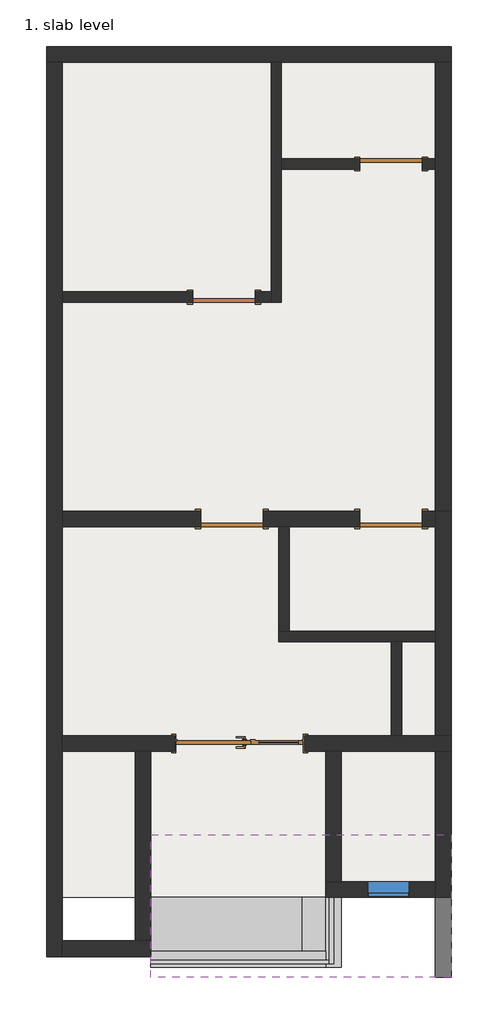
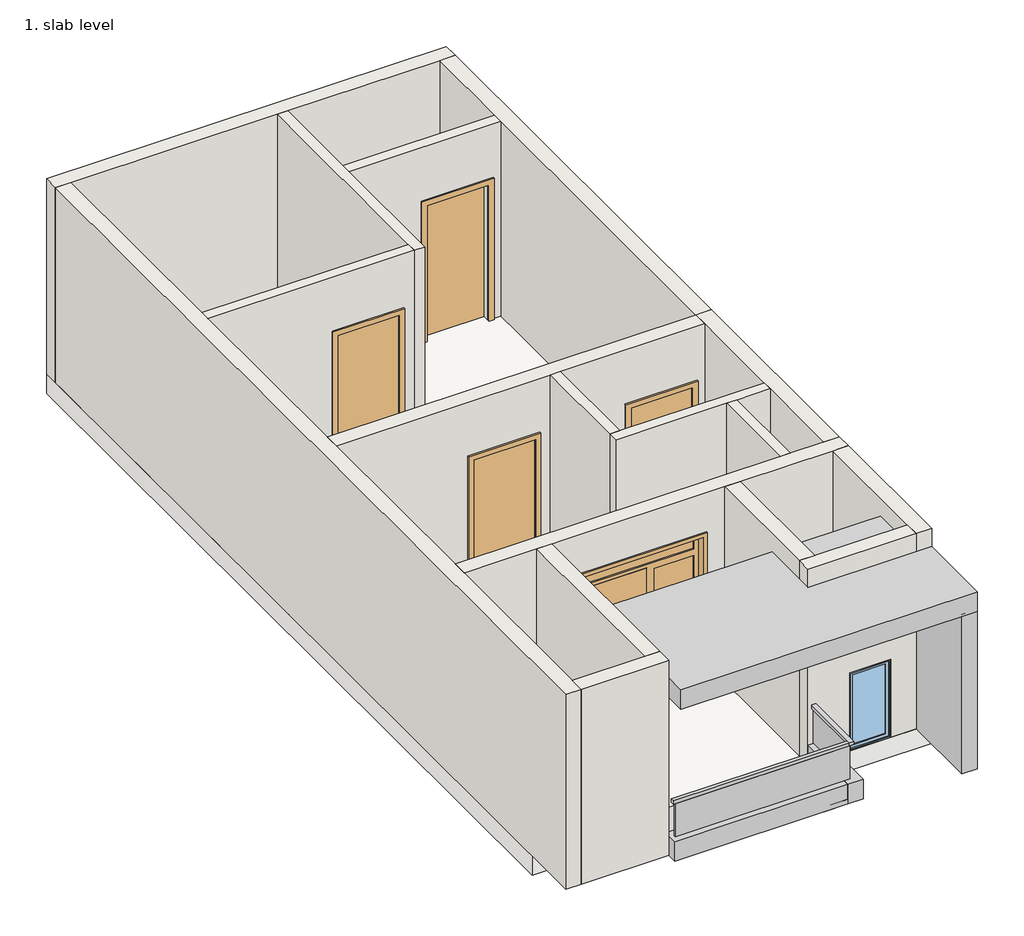
# One storey: 17 walls, 6 proxies, 5 doors, 1 slab, 1 window.
"""IFC4 building model written with IfcOpenShell, lengths in millimetres."""

from ifc_helpers import new_model, si_unit, frame, origin, place, context, project, spatial, polyline, outline, extrude, faceted_brep, transform, mapped, element, save
from components import generic_models_11_generic_models_11_7edcfdbd, generic_models_13_generic_models_13_04127036, generic_models_14_generic_models_14_d7e62491, generic_models_6_generic_models_6_4fc6bb2b, generic_models_8_generic_models_8_7572a94e, generic_models_9_generic_models_9_4d3f9729, main_entrance_door_11153_main_entrance_door_11153_94c2f9e1, door_686f89d2, door_a90ba1ad, fixed_2_x3_c82808a1

model = new_model("IFC4")

# Units and contexts
model_context = context("Model", 3, world=origin())
ifc_project = project(units=[si_unit("LENGTHUNIT", "METRE", prefix="MILLI")], contexts=[model_context])

# Site, building, storey
site = spatial("IfcSite", under=ifc_project)
building = spatial("IfcBuilding", under=site)
storey = spatial("IfcBuildingStorey", under=building, Name="1. slab level", Elevation=3657.6)

# Proxies
placement = place(None, origin())
generic_models_11_generic_models_11_shape = generic_models_11_generic_models_11_7edcfdbd(model_context)
element("IfcBuildingElementProxy", 1, Name="Generic Models 11 : Generic Models 11", ObjectType="Generic Models 11 : Generic Models 11", at=placement, inside=storey, context=model_context, shape_type="MappedRepresentation", body=[
    mapped(generic_models_11_generic_models_11_shape, transform((0.0, 0.0, 0.0), x_axis=(1.0, 0.0, 0.0), y_axis=(0.0, 1.0, 0.0), z_axis=(0.0, 0.0, 1.0))),
])
generic_models_13_generic_models_13_shape = generic_models_13_generic_models_13_04127036(model_context)
element("IfcBuildingElementProxy", 2, Name="Generic Models 13 : Generic Models 13", ObjectType="Generic Models 13 : Generic Models 13", at=placement, inside=storey, context=model_context, shape_type="MappedRepresentation", body=[
    mapped(generic_models_13_generic_models_13_shape, transform((0.0, 0.0, 0.0), x_axis=(1.0, 0.0, 0.0), y_axis=(0.0, 1.0, 0.0), z_axis=(0.0, 0.0, 1.0))),
])
generic_models_14_generic_models_14_shape = generic_models_14_generic_models_14_d7e62491(model_context)
element("IfcBuildingElementProxy", 3, Name="Generic Models 14 : Generic Models 14", ObjectType="Generic Models 14 : Generic Models 14", at=placement, inside=storey, context=model_context, shape_type="MappedRepresentation", body=[
    mapped(generic_models_14_generic_models_14_shape, transform((0.0, 0.0, 0.0), x_axis=(1.0, 0.0, 0.0), y_axis=(0.0, 1.0, 0.0), z_axis=(0.0, 0.0, 1.0))),
])
generic_models_6_generic_models_6_shape = generic_models_6_generic_models_6_4fc6bb2b(model_context)
element("IfcBuildingElementProxy", 4, Name="Generic Models 6 : Generic Models 6", ObjectType="Generic Models 6 : Generic Models 6", at=placement, inside=storey, context=model_context, shape_type="MappedRepresentation", body=[
    mapped(generic_models_6_generic_models_6_shape, transform((0.0, 0.0, 0.0), x_axis=(1.0, 0.0, 0.0), y_axis=(0.0, 1.0, 0.0), z_axis=(0.0, 0.0, 1.0))),
])
generic_models_8_generic_models_8_shape = generic_models_8_generic_models_8_7572a94e(model_context)
element("IfcBuildingElementProxy", 5, Name="Generic Models 8 : Generic Models 8", ObjectType="Generic Models 8 : Generic Models 8", at=placement, inside=storey, context=model_context, shape_type="MappedRepresentation", body=[
    mapped(generic_models_8_generic_models_8_shape, transform((0.0, 0.0, 0.0), x_axis=(1.0, 0.0, 0.0), y_axis=(0.0, 1.0, 0.0), z_axis=(0.0, 0.0, 1.0))),
])
generic_models_9_generic_models_9_shape = generic_models_9_generic_models_9_4d3f9729(model_context)
element("IfcBuildingElementProxy", 6, Name="Generic Models 9 : Generic Models 9", ObjectType="Generic Models 9 : Generic Models 9", at=placement, inside=storey, context=model_context, shape_type="MappedRepresentation", body=[
    mapped(generic_models_9_generic_models_9_shape, transform((0.0, 0.0, 0.0), x_axis=(1.0, 0.0, 0.0), y_axis=(0.0, 1.0, 0.0), z_axis=(0.0, 0.0, 1.0))),
])

# Doors
main_entrance_door_11153_main_entrance_door_11153_shape = main_entrance_door_11153_main_entrance_door_11153_94c2f9e1(model_context)
element("IfcDoor", 7, ObjectType="Main_entrance_door_11153 : Main_entrance_door_11153", at=placement, inside=storey, context=model_context, shape_type="MappedRepresentation", body=[
    mapped(main_entrance_door_11153_main_entrance_door_11153_shape, transform((-13607.1371373, -268.761407, 3657.6), x_axis=(1.0, 0.0, 0.0), y_axis=(0.0, 1.0, 0.0), z_axis=(0.0, 0.0, 1.0))),
])
door_shape = door_686f89d2(model_context)
element("IfcDoor", 8, ObjectType="Single-Flush : 36\" x 84\"", at=placement, inside=storey, context=model_context, shape_type="MappedRepresentation", body=[
    mapped(door_shape, transform((-13835.7371373, 6246.338593, 3657.6), x_axis=(1.0, 0.0, 0.0), y_axis=(0.0, 1.0, 0.0), z_axis=(0.0, 0.0, 1.0))),
])
element("IfcDoor", 9, ObjectType="Single-Flush : 36\" x 84\"", at=placement, inside=storey, context=model_context, shape_type="MappedRepresentation", body=[
    mapped(door_shape, transform((-11397.3371373, 8189.438593, 3657.6), x_axis=(-1.0, 0.0, 0.0), y_axis=(0.0, -1.0, 0.0), z_axis=(0.0, 0.0, 1.0))),
])
door_2_shape = door_a90ba1ad(model_context)
element("IfcDoor", 10, ObjectType="Single-Flush : 36\" x 84\"", at=placement, inside=storey, context=model_context, shape_type="MappedRepresentation", body=[
    mapped(door_2_shape, transform((-13721.4371373, 3007.838593, 3657.6), x_axis=(1.0, 0.0, 0.0), y_axis=(0.0, 1.0, 0.0), z_axis=(0.0, 0.0, 1.0))),
])
element("IfcDoor", 11, ObjectType="Single-Flush : 36\" x 84\"", at=placement, inside=storey, context=model_context, shape_type="MappedRepresentation", body=[
    mapped(door_2_shape, transform((-11397.3371373, 3007.838593, 3657.6), x_axis=(1.0, 0.0, 0.0), y_axis=(0.0, 1.0, 0.0), z_axis=(0.0, 0.0, 1.0))),
])

# Slab
element("IfcSlab", 12, ObjectType="slab 6\"", at=placement, inside=storey, context=model_context, shape_type="SweptSolid", body=[
    extrude(outline(polyline([(-10521.0371373, 9903.938593), (-10521.0371373, -2516.661407), (-16426.5371373, -2516.661407), (-16426.5371373, 9903.938593), (-10521.0371373, 9903.938593)])), frame((0.0, 0.0, 3352.8), z_axis=(0.0, 0.0, 1.0), x_axis=(1.0, 0.0, 0.0)), (0.0, 0.0, 1.0), 304.8),
])

# Walls
element("IfcWall", 13, ObjectType="wall 6\"", at=placement, inside=storey, context=model_context, shape_type="Brep", body=[
    faceted_brep([(-13149.9371373, 9675.338593, 3657.6), (-13149.9371373, 6322.538593, 3657.6), (-13149.9371373, 6170.138593, 3657.6), (-13149.9371373, 6170.138593, 6705.6), (-13149.9371373, 6322.538593, 6705.6), (-13149.9371373, 9675.338593, 6705.6), (-12997.5371373, 9675.338593, 3657.6), (-12997.5371373, 9675.338593, 6705.6), (-12997.5371373, 8265.638593, 6705.6), (-12997.5371373, 8113.238593, 6705.6), (-12997.5371373, 6170.138593, 6705.6), (-12997.5371373, 6170.138593, 3657.6), (-12997.5371373, 8113.238593, 3657.6), (-12997.5371373, 8265.638593, 3657.6)], [[[0, 1, 2, 3, 4, 5]], [[6, 7, 8, 9, 10, 11, 12, 13]], [[2, 1, 0, 6, 13, 12, 11]], [[5, 4, 3, 10, 9, 8, 7]], [[0, 5, 7, 6]], [[3, 2, 11, 10]]]),
])
element("IfcWall", 14, ObjectType="wall 6\"", at=placement, inside=storey, context=model_context, shape_type="SweptSolid", body=[
    extrude(outline(polyline([(5791.2, -13378.5371373), (3657.6, -13378.5371373), (3657.6, -13149.9371373), (6705.6, -13149.9371373), (6705.6, -16197.9371373), (3657.6, -16197.9371373), (3657.6, -14292.9371373), (5791.2, -14292.9371373), (5791.2, -13378.5371373)])), frame((0.0, 6170.138593, 0.0), z_axis=(0.0, 1.0, 0.0), x_axis=(0.0, 0.0, 1.0)), (0.0, 0.0, 1.0), 152.4),
])
element("IfcWall", 15, ObjectType="wall 6\"", at=placement, inside=storey, context=model_context, shape_type="SweptSolid", body=[
    extrude(outline(polyline([(3657.6, -12997.5371373), (3657.6, -11854.5371373), (5791.2, -11854.5371373), (5791.2, -10940.1371373), (3657.6, -10940.1371373), (3657.6, -10749.6371373), (6705.6, -10749.6371373), (6705.6, -12997.5371373), (3657.6, -12997.5371373)])), frame((0.0, 8113.238593, 0.0), z_axis=(0.0, 1.0, 0.0), x_axis=(0.0, 0.0, 1.0)), (0.0, 0.0, 1.0), 152.4),
])
element("IfcWall", 16, ObjectType="wall 6\"", at=placement, inside=storey, context=model_context, shape_type="Brep", body=[
    faceted_brep([(-10749.6371373, 1369.538593, 3657.6), (-12883.2371373, 1369.538593, 3657.6), (-13035.6371373, 1369.538593, 3657.6), (-13035.6371373, 1369.538593, 6705.6), (-12883.2371373, 1369.538593, 6705.6), (-10749.6371373, 1369.538593, 6705.6), (-10749.6371373, 1217.138593, 3657.6), (-10749.6371373, 1217.138593, 6705.6), (-11244.9371373, 1217.138593, 6705.6), (-11397.3371373, 1217.138593, 6705.6), (-13035.6371373, 1217.138593, 6705.6), (-13035.6371373, 1217.138593, 3657.6), (-11397.3371373, 1217.138593, 3657.6), (-11244.9371373, 1217.138593, 3657.6)], [[[0, 1, 2, 3, 4, 5]], [[6, 7, 8, 9, 10, 11, 12, 13]], [[2, 1, 0, 6, 13, 12, 11]], [[5, 4, 3, 10, 9, 8, 7]], [[0, 5, 7, 6]], [[3, 2, 11, 10]]]),
])
element("IfcWall", 17, ObjectType="wall 6\"", at=placement, inside=storey, context=model_context, shape_type="SweptSolid", body=[
    extrude(outline(polyline([(-12883.2371373, 2893.538593), (-12883.2371373, 1369.538593), (-13035.6371373, 1369.538593), (-13035.6371373, 2893.538593), (-12883.2371373, 2893.538593)])), frame((0.0, 0.0, 3657.6), z_axis=(0.0, 0.0, 1.0), x_axis=(1.0, 0.0, 0.0)), (0.0, 0.0, 1.0), 3048.0),
])
element("IfcWall", 18, ObjectType="wall 6\"", at=placement, inside=storey, context=model_context, shape_type="SweptSolid", body=[
    extrude(outline(polyline([(-11397.3371373, -154.461407), (-11397.3371373, 1217.138593), (-11244.9371373, 1217.138593), (-11244.9371373, -154.461407), (-11397.3371373, -154.461407)])), frame((0.0, 0.0, 3657.6), z_axis=(0.0, 0.0, 1.0), x_axis=(1.0, 0.0, 0.0)), (0.0, 0.0, 1.0), 3048.0),
])
element("IfcWall", 19, ObjectType="wall 9\"", at=placement, inside=storey, context=model_context, shape_type="Brep", body=[
    faceted_brep([(-16426.5371373, 9675.338593, 3657.6), (-16197.9371373, 9675.338593, 3657.6), (-13149.9371373, 9675.338593, 3657.6), (-12997.5371373, 9675.338593, 3657.6), (-10749.6371373, 9675.338593, 3657.6), (-10521.0371373, 9675.338593, 3657.6), (-10521.0371373, 9675.338593, 6705.6), (-10749.6371373, 9675.338593, 6705.6), (-12997.5371373, 9675.338593, 6705.6), (-13149.9371373, 9675.338593, 6705.6), (-16197.9371373, 9675.338593, 6705.6), (-16426.5371373, 9675.338593, 6705.6), (-16426.5371373, 9903.938593, 3657.6), (-16426.5371373, 9903.938593, 6705.6), (-10521.0371373, 9903.938593, 6705.6), (-10521.0371373, 9903.938593, 3657.6)], [[[0, 1, 2, 3, 4, 5, 6, 7, 8, 9, 10, 11]], [[12, 13, 14, 15]], [[5, 4, 3, 2, 1, 0, 12, 15]], [[11, 10, 9, 8, 7, 6, 14, 13]], [[0, 11, 13, 12]], [[6, 5, 15, 14]]]),
])
element("IfcWall", 20, ObjectType="wall 9\"", at=placement, inside=storey, context=model_context, shape_type="Brep", body=[
    faceted_brep([(-16426.5371373, 9675.338593, 3657.6), (-16426.5371373, -3380.261407, 3657.6), (-16426.5371373, -3380.261407, 6705.6), (-16426.5371373, 9675.338593, 6705.6), (-16197.9371373, 9675.338593, 3657.6), (-16197.9371373, 9675.338593, 6705.6), (-16197.9371373, 6322.538593, 6705.6), (-16197.9371373, 6170.138593, 6705.6), (-16197.9371373, 3122.138593, 6705.6), (-16197.9371373, 2893.538593, 6705.6), (-16197.9371373, -154.461407, 6705.6), (-16197.9371373, -383.061407, 6705.6), (-16197.9371373, -3151.661407, 6705.6), (-16197.9371373, -3380.261407, 6705.6), (-16197.9371373, -3380.261407, 3657.6), (-16197.9371373, -3151.661407, 3657.6), (-16197.9371373, -383.061407, 3657.6), (-16197.9371373, -154.461407, 3657.6), (-16197.9371373, 2893.538593, 3657.6), (-16197.9371373, 3122.138593, 3657.6), (-16197.9371373, 6170.138593, 3657.6), (-16197.9371373, 6322.538593, 3657.6)], [[[0, 1, 2, 3]], [[4, 5, 6, 7, 8, 9, 10, 11, 12, 13, 14, 15, 16, 17, 18, 19, 20, 21]], [[1, 0, 4, 21, 20, 19, 18, 17, 16, 15, 14]], [[3, 2, 13, 12, 11, 10, 9, 8, 7, 6, 5]], [[0, 3, 5, 4]], [[2, 1, 14, 13]]]),
])
element("IfcWall", 21, ObjectType="wall 9\"", at=placement, inside=storey, context=model_context, shape_type="Brep", body=[
    faceted_brep([(-10940.1371373, 2893.538593, 5791.2), (-10940.1371373, 2893.538593, 3657.6), (-10749.6371373, 2893.538593, 3657.6), (-10749.6371373, 2893.538593, 6705.6), (-12883.2371373, 2893.538593, 6705.6), (-13035.6371373, 2893.538593, 6705.6), (-16197.9371373, 2893.538593, 6705.6), (-16197.9371373, 2893.538593, 3657.6), (-14178.6371373, 2893.538593, 3657.6), (-14178.6371373, 2893.538593, 5791.2), (-13264.2371373, 2893.538593, 5791.2), (-13264.2371373, 2893.538593, 3657.6), (-13035.6371373, 2893.538593, 3657.6), (-12883.2371373, 2893.538593, 3657.6), (-11854.5371373, 2893.538593, 3657.6), (-11854.5371373, 2893.538593, 5791.2), (-10749.6371373, 3122.138593, 3657.6), (-10940.1371373, 3122.138593, 3657.6), (-10940.1371373, 3122.138593, 5791.2), (-11854.5371373, 3122.138593, 5791.2), (-11854.5371373, 3122.138593, 3657.6), (-13264.2371373, 3122.138593, 3657.6), (-13264.2371373, 3122.138593, 5791.2), (-14178.6371373, 3122.138593, 5791.2), (-14178.6371373, 3122.138593, 3657.6), (-16197.9371373, 3122.138593, 3657.6), (-16197.9371373, 3122.138593, 6705.6), (-10749.6371373, 3122.138593, 6705.6)], [[[0, 1, 2, 3, 4, 5, 6, 7, 8, 9, 10, 11, 12, 13, 14, 15]], [[16, 17, 18, 19, 20, 21, 22, 23, 24, 25, 26, 27]], [[8, 7, 25, 24]], [[2, 1, 17, 16]], [[14, 13, 12, 11, 21, 20]], [[6, 5, 4, 3, 27, 26]], [[7, 6, 26, 25]], [[3, 2, 16, 27]], [[22, 21, 11, 10]], [[23, 22, 10, 9]], [[24, 23, 9, 8]], [[18, 17, 1, 0]], [[19, 18, 0, 15]], [[20, 19, 15, 14]]]),
])
element("IfcWall", 22, ObjectType="wall 9\"", at=placement, inside=storey, context=model_context, shape_type="Brep", body=[
    faceted_brep([(-10749.6371373, 9675.338593, 3657.6), (-10749.6371373, 8265.638593, 3657.6), (-10749.6371373, 8113.238593, 3657.6), (-10749.6371373, 3122.138593, 3657.6), (-10749.6371373, 3122.138593, 6705.6), (-10749.6371373, 8113.238593, 6705.6), (-10749.6371373, 8265.638593, 6705.6), (-10749.6371373, 9675.338593, 6705.6), (-10521.0371373, 9675.338593, 3657.6), (-10521.0371373, 9675.338593, 6705.6), (-10521.0371373, 3122.138593, 6705.6), (-10521.0371373, 3122.138593, 3657.6)], [[[0, 1, 2, 3, 4, 5, 6, 7]], [[8, 9, 10, 11]], [[3, 2, 1, 0, 8, 11]], [[7, 6, 5, 4, 10, 9]], [[0, 7, 9, 8]], [[4, 3, 11, 10]]]),
])
element("IfcWall", 23, ObjectType="wall 9\"", at=placement, inside=storey, context=model_context, shape_type="Brep", body=[
    faceted_brep([(-10521.0371373, -383.061407, 6705.6), (-10749.6371373, -383.061407, 6705.6), (-12121.2371373, -383.061407, 6705.6), (-12349.8371373, -383.061407, 6705.6), (-14902.5371373, -383.061407, 6705.6), (-15131.1371373, -383.061407, 6705.6), (-16197.9371373, -383.061407, 6705.6), (-16197.9371373, -383.061407, 3657.6), (-15131.1371373, -383.061407, 3657.6), (-14902.5371373, -383.061407, 3657.6), (-14557.1371373, -383.061407, 3657.6), (-14557.1371373, -383.061407, 6057.6), (-12657.1371373, -383.061407, 6057.6), (-12657.1371373, -383.061407, 3657.6), (-12349.8371373, -383.061407, 3657.6), (-12121.2371373, -383.061407, 3657.6), (-10749.6371373, -383.061407, 3657.6), (-10521.0371373, -383.061407, 3657.6), (-16197.9371373, -154.461407, 6705.6), (-11397.3371373, -154.461407, 6705.6), (-11244.9371373, -154.461407, 6705.6), (-10749.6371373, -154.461407, 6705.6), (-10521.0371373, -154.461407, 6705.6), (-10521.0371373, -154.461407, 3657.6), (-10749.6371373, -154.461407, 3657.6), (-11244.9371373, -154.461407, 3657.6), (-11397.3371373, -154.461407, 3657.6), (-12657.1371373, -154.461407, 3657.6), (-12657.1371373, -154.461407, 6057.6), (-14557.1371373, -154.461407, 6057.6), (-14557.1371373, -154.461407, 3657.6), (-16197.9371373, -154.461407, 3657.6)], [[[0, 1, 2, 3, 4, 5, 6, 7, 8, 9, 10, 11, 12, 13, 14, 15, 16, 17]], [[18, 19, 20, 21, 22, 23, 24, 25, 26, 27, 28, 29, 30, 31]], [[7, 31, 30, 10, 9, 8]], [[23, 17, 16, 15, 14, 13, 27, 26, 25, 24]], [[6, 5, 4, 3, 2, 1, 0, 22, 21, 20, 19, 18]], [[7, 6, 18, 31]], [[0, 17, 23, 22]], [[12, 28, 27, 13]], [[28, 12, 11, 29]], [[29, 11, 10, 30]]]),
])
element("IfcWall", 24, ObjectType="wall 9\"", at=placement, inside=storey, context=model_context, shape_type="Brep", body=[
    faceted_brep([(-10521.0371373, -154.461407, 3657.6), (-10521.0371373, 3122.138593, 3657.6), (-10521.0371373, 3122.138593, 6705.6), (-10521.0371373, -154.461407, 6705.6), (-10749.6371373, -154.461407, 3657.6), (-10749.6371373, -154.461407, 6705.6), (-10749.6371373, 1217.138593, 6705.6), (-10749.6371373, 1369.538593, 6705.6), (-10749.6371373, 2893.538593, 6705.6), (-10749.6371373, 3122.138593, 6705.6), (-10749.6371373, 3122.138593, 3657.6), (-10749.6371373, 2893.538593, 3657.6), (-10749.6371373, 1369.538593, 3657.6), (-10749.6371373, 1217.138593, 3657.6)], [[[0, 1, 2, 3]], [[4, 5, 6, 7, 8, 9, 10, 11, 12, 13]], [[1, 0, 4, 13, 12, 11, 10]], [[3, 2, 9, 8, 7, 6, 5]], [[0, 3, 5, 4]], [[2, 1, 10, 9]]]),
])
element("IfcWall", 25, ObjectType="wall 9\"", at=placement, inside=storey, context=model_context, shape_type="Brep", body=[
    faceted_brep([(-10749.6371373, -383.061407, 3657.6), (-10749.6371373, -2288.061407, 3657.6), (-10749.6371373, -2516.661407, 3657.6), (-10749.6371373, -2516.661407, 6705.6), (-10749.6371373, -2288.061407, 6705.6), (-10749.6371373, -383.061407, 6705.6), (-10521.0371373, -383.061407, 3657.6), (-10521.0371373, -383.061407, 6705.6), (-10521.0371373, -2516.661407, 6705.6), (-10521.0371373, -2516.661407, 3657.6)], [[[0, 1, 2, 3, 4, 5]], [[6, 7, 8, 9]], [[2, 1, 0, 6, 9]], [[5, 4, 3, 8, 7]], [[0, 5, 7, 6]], [[3, 2, 9, 8]]]),
])
element("IfcWall", 26, ObjectType="wall 9\"", at=placement, inside=storey, context=model_context, shape_type="SweptSolid", body=[
    extrude(outline(polyline([(-12121.2371373, -383.061407), (-12121.2371373, -2288.061407), (-12349.8371373, -2288.061407), (-12349.8371373, -383.061407), (-12121.2371373, -383.061407)])), frame((0.0, 0.0, 3657.6), z_axis=(0.0, 0.0, 1.0), x_axis=(1.0, 0.0, 0.0)), (0.0, 0.0, 1.0), 3048.0),
])
element("IfcWall", 27, ObjectType="wall 9\"", at=placement, inside=storey, context=model_context, shape_type="Brep", body=[
    faceted_brep([(-16197.9371373, -3380.261407, 3657.6), (-14902.5371373, -3380.261407, 3657.6), (-14902.5371373, -3380.261407, 6705.6), (-16197.9371373, -3380.261407, 6705.6), (-16197.9371373, -3151.661407, 3657.6), (-16197.9371373, -3151.661407, 6705.6), (-15131.1371373, -3151.661407, 6705.6), (-14902.5371373, -3151.661407, 6705.6), (-14902.5371373, -3151.661407, 3657.6), (-15131.1371373, -3151.661407, 3657.6)], [[[0, 1, 2, 3]], [[4, 5, 6, 7, 8, 9]], [[1, 0, 4, 9, 8]], [[3, 2, 7, 6, 5]], [[0, 3, 5, 4]], [[2, 1, 8, 7]]]),
])
element("IfcWall", 28, ObjectType="wall 9\"", at=placement, inside=storey, context=model_context, shape_type="SweptSolid", body=[
    extrude(outline(polyline([(-14902.5371373, -383.061407), (-14902.5371373, -3151.661407), (-15131.1371373, -3151.661407), (-15131.1371373, -383.061407), (-14902.5371373, -383.061407)])), frame((0.0, 0.0, 3657.6), z_axis=(0.0, 0.0, 1.0), x_axis=(1.0, 0.0, 0.0)), (0.0, 0.0, 1.0), 3048.0),
])
element("IfcWall", 29, ObjectType="wall 9\"", at=placement, inside=storey, context=model_context, shape_type="Brep", body=[
    faceted_brep([(-12349.8371373, -2288.061407, 6705.6), (-12121.2371373, -2288.061407, 6705.6), (-10749.6371373, -2288.061407, 6705.6), (-10749.6371373, -2288.061407, 3657.6), (-11130.6371373, -2288.061407, 3657.6), (-11130.6371373, -2288.061407, 4876.8), (-11740.2371373, -2288.061407, 4876.8), (-11740.2371373, -2288.061407, 3657.6), (-12121.2371373, -2288.061407, 3657.6), (-12349.8371373, -2288.061407, 3657.6), (-10749.6371373, -2516.661407, 6705.6), (-12349.8371373, -2516.661407, 6705.6), (-12349.8371373, -2516.661407, 3657.6), (-11740.2371373, -2516.661407, 3657.6), (-11740.2371373, -2516.661407, 4876.8), (-11130.6371373, -2516.661407, 4876.8), (-11130.6371373, -2516.661407, 3657.6), (-10749.6371373, -2516.661407, 3657.6)], [[[0, 1, 2, 3, 4, 5, 6, 7, 8, 9]], [[10, 11, 12, 13, 14, 15, 16, 17]], [[3, 17, 16, 4]], [[12, 9, 8, 7, 13]], [[2, 1, 0, 11, 10]], [[3, 2, 10, 17]], [[0, 9, 12, 11]], [[6, 14, 13, 7]], [[15, 5, 4, 16]], [[14, 6, 5, 15]]]),
])

# Window
fixed_2_x3_shape = fixed_2_x3_c82808a1(model_context)
element("IfcWindow", 30, ObjectType="Fixed : 2'X3'", at=placement, inside=storey, context=model_context, shape_type="MappedRepresentation", body=[
    mapped(fixed_2_x3_shape, transform((-11473.5371373, -2402.361407, 2743.2), x_axis=(-1.0, 0.0, 0.0), y_axis=(0.0, -1.0, 0.0), z_axis=(0.0, 0.0, 1.0))),
])

save(model, "model.ifc")

# Revit data of these elements
# Type "Main_entrance_door_11153 : Main_entrance_door_11153"
#   Type Mark = "8"
#   Height = 7' - 10.48819"
#   Width = 6' - 2.80315"
#   Door Width = 3' - 7.30709"
#   Function = (empty or 0)
#   Wall Closure = (empty or 0)
# Type "Single-Flush : 36\" x 84\""
#   Type Mark = "1"
#   Construction Type Id = "MDOOR"
#   Assembly Code = "C1020"
#   Analytic Construction = "Metal"
#   Thickness = 0' - 2"
#   Heat Transfer Coefficient (U) = 0.651978 BTU/(h·ft²·°F)
#   Height = 7' - 0"
#   Trim Projection Ext = 0' - 1"
#   Trim Projection Int = 0' - 1"
#   Trim Width = 0' - 3"
#   Width = 3' - 0"
#   Define Thermal Properties by = 1
#   Define Thermal Properties by = 1
#   Door Material = Door - Panel
#   Frame Material = Door - Frame
#   Visual Light Transmittance = 0
#   Solar Heat Gain Coefficient = 0
#   Function = (empty or 0)
#   Wall Closure = (empty or 0)
# Type "slab 6\""
#   Assembly Code = "B1010"
#   Function = 0
#   Layers, outside or top first: 1' - 0" no material (function 1)
# Type "wall 6\""
#   Assembly Code = "B2010"
#   Layers, outside or top first: 0' - 6" no material (function 1)
# Type "wall 9\""
#   Assembly Code = "B2010"
#   Layers, outside or top first: 0' - 9" no material (function 1)
# Type "Fixed : 2'X3'"
#   Type Mark = "19"
#   Construction Type Id = "GSP4R"
#   Assembly Code = "B2020100"
#   Analytic Construction = "1/8 in Pilkington single glazing"
#   Visual Light Transmittance = 0.9
#   Solar Heat Gain Coefficient = 0.78
#   Heat Transfer Coefficient (U) = 0.6496 BTU/(h·ft²·°F)
#   Height = 4' - 0"
#   Default Sill Height = 3' - 0"
#   Width = 2' - 0"
#   Window Inset = 0' - 0 3/4"
#   Define Thermal Properties by = 1
#   Glass Pane Material = Glass
#   Sash Material = Sash
#   Wall Closure = (empty or 0)
# Element 1 (IfcBuildingElementProxy, "Generic Models 11 : Generic Models 11")
#   Phase Created = New Construction
#   Materials on its faces: "Gypsum Wall Board"
# Element 2 (IfcBuildingElementProxy, "Generic Models 13 : Generic Models 13")
#   Phase Created = New Construction
#   Materials on its faces: "Steel, Carbon", "Steel, Chrome Plated"
# Element 3 (IfcBuildingElementProxy, "Generic Models 14 : Generic Models 14")
#   Phase Created = New Construction
#   Materials on its faces: "Default Mass Interior Wall", "Default Form"
# Element 4 (IfcBuildingElementProxy, "Generic Models 6 : Generic Models 6")
#   Phase Created = New Construction
#   Materials on its faces: "Gypsum Wall Board"
# Element 5 (IfcBuildingElementProxy, "Generic Models 8 : Generic Models 8")
#   Phase Created = New Construction
#   Materials on its faces: "Gypsum Wall Board"
# Element 6 (IfcBuildingElementProxy, "Generic Models 9 : Generic Models 9")
#   Phase Created = New Construction
#   Materials on its faces: "Gypsum Wall Board"
# Element 7 (IfcDoor, "Main_entrance_door_11153 : Main_entrance_door_11153")
#   Phase Created = New Construction
#   Materials on its faces: "Glass", "Default"
# Elements 8, 9, 10, 11 (IfcDoor, "Single-Flush : 36\" x 84\"")
#   Phase Created = New Construction
#   Materials on its faces: "Door - Frame", "Door - Panel"
# Element 12 (IfcSlab, "slab 6\"")
#   Height Offset From Level = 0' - 0"
#   Phase Created = New Construction
#   Materials on its faces: "1. WALL PAINT", "Default Floor", "5. GRAVEL"
# Elements 13, 14, 15, 16, 17 (IfcWall, "wall 6\"")
#   Top Offset = 0' - 0"
#   Base Offset = 0' - 0"
#   wall height = 10' - 0"
#   Phase Created = New Construction
#   Base Constraint = 1. slab level
#   Top Constraint = first floor slab
#   Materials on its faces: "Default Wall"
# Element 18 (IfcWall, "wall 6\"")
#   Top Offset = 0' - 0"
#   Base Offset = 0' - 0"
#   wall height = 10' - 0"
#   Phase Created = New Construction
#   Base Constraint = 1. slab level
#   Top Constraint = first floor slab
#   Materials on its faces: "Default Wall", "Laminate, Ivory, Matte"
# Elements 19, 20, 22, 24 (IfcWall, "wall 9\"")
#   Top Offset = 0' - 0"
#   Base Offset = 0' - 0"
#   wall height = 10' - 0"
#   Phase Created = New Construction
#   Base Constraint = 1. slab level
#   Top Constraint = first floor slab
#   Materials on its faces: "Default Wall", "4. WALL PAINT"
# Element 21 (IfcWall, "wall 9\"")
#   Top Offset = 0' - 0"
#   Base Offset = 0' - 0"
#   wall height = 10' - 0"
#   Phase Created = New Construction
#   Base Constraint = 1. slab level
#   Top Constraint = first floor slab
#   Materials on its faces: "Default Wall"
# Element 23 (IfcWall, "wall 9\"")
#   Top Offset = 0' - 0"
#   Base Offset = 0' - 0"
#   wall height = 10' - 0"
#   Phase Created = New Construction
#   Base Constraint = 1. slab level
#   Top Constraint = first floor slab
#   Materials on its faces: "Default Wall", "3. wall paint", "4. WALL PAINT"
# Element 25 (IfcWall, "wall 9\"")
#   Top Offset = 0' - 0"
#   Base Offset = 0' - 0"
#   wall height = 10' - 0"
#   Phase Created = New Construction
#   Base Constraint = 1. slab level
#   Top Constraint = first floor slab
#   Materials on its faces: "Tile, Porcelain, 4in", "Default Wall", "4. WALL PAINT", "Wood Planks"
# Elements 26, 27, 28 (IfcWall, "wall 9\"")
#   Top Offset = 0' - 0"
#   Base Offset = 0' - 0"
#   wall height = 10' - 0"
#   Phase Created = New Construction
#   Base Constraint = 1. slab level
#   Top Constraint = first floor slab
#   Materials on its faces: "Default Wall", "3. wall paint"
# Element 29 (IfcWall, "wall 9\"")
#   Top Offset = 0' - 0"
#   Base Offset = 0' - 0"
#   wall height = 10' - 0"
#   Phase Created = New Construction
#   Base Constraint = 1. slab level
#   Top Constraint = first floor slab
#   Materials on its faces: "Default Wall", "Wood Planks", "3. wall paint"
# Element 30 (IfcWindow, "Fixed : 2'X3'")
#   Mark = "9"
#   Phase Created = New Construction
#   Materials on its faces: "Sash", "Glass"
# Materials
#   "Door - Panel": class "Wood", colour RGB 210 159 95, transparency 0, Cost = 0
#   "Door - Frame": colour RGB 118 70 51, transparency 0, Cost = 0
#   "Glass": class "Glass", colour RGB 0 128 192, transparency 0.75, Description = "Soda Lime Glass", Cost = 0
#   "Sash": class "Wood", colour RGB 224 178 126, transparency 0, Cost = 0
#   "Gypsum Wall Board": class "Generic", colour RGB 127 127 127, transparency 0, Description = "Gypsum Wall Board", Cost = 0
#   "Steel, Carbon": class "Metal", colour RGB 0 0 0, transparency 0, Description = "Carbon steel", Cost = 0
#   "Steel, Chrome Plated": class "Metal", colour RGB 17 17 17, transparency 0, Description = "Chromiuim plated steel", Cost = 0
#   "Default Mass Interior Wall": class "Generic", colour RGB 195 229 126, transparency 0, Cost = 0
#   "Default Form": class "Generic", colour RGB 185 189 196, transparency 0.5, Cost = 0
#   "Default": colour RGB 127 127 127, transparency 0, Cost = 0
#   "1. WALL PAINT": class "Generic", colour RGB 120 120 120, transparency 0, Cost = 0
#   "Default Floor": colour RGB 128 128 128, transparency 0, Cost = 0
#   "5. GRAVEL": class "Generic", colour RGB 120 120 120, transparency 0, Cost = 0
#   "Default Wall": colour RGB 128 128 128, transparency 0, Cost = 0
#   "Laminate, Ivory, Matte": class "Plastic", colour RGB 247 247 239, transparency 0, Description = "Plastic Laminate - Ivory, Matte", Cost = 0
#   "4. WALL PAINT": class "Generic", colour RGB 120 120 120, transparency 0, Cost = 0
#   "3. wall paint": class "Generic", colour RGB 120 120 120, transparency 0, Cost = 0
#   "Tile, Porcelain, 4in": class "Generic", colour RGB 89 87 158, transparency 0, Description = "Porcelain tile, 4\", white", Cost = 0
#   "Wood Planks": class "Wood", colour RGB 193 160 115, transparency 0, Description = "Physical material.", Cost = 0
